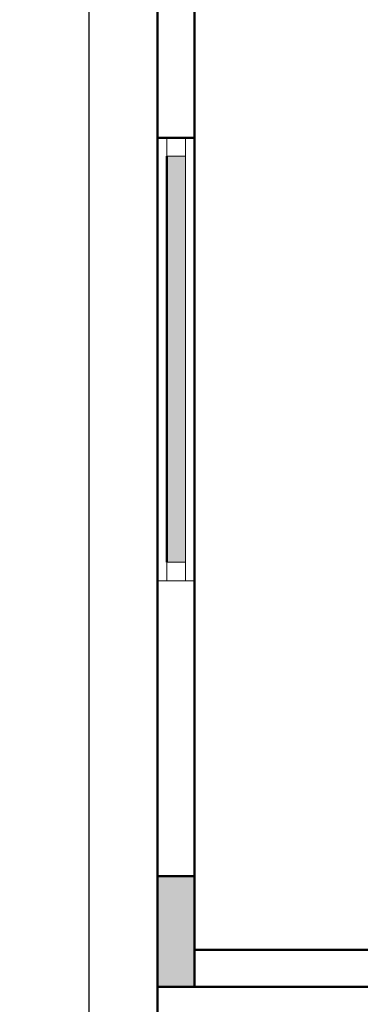
# Model space of a CAD drawing. Units: inches. Extents: x 3064 to 19385, y 846 to 15425.
# Tile 11 of 108: x 3625 to 3680, y 974 to 1134. Entities that reach past the tile are written whole.
import ezdxf

# ---------------------------------------------------------------- set-up
doc = ezdxf.new("R2010")
doc.units = ezdxf.units.IN
for name, color, linetype, lineweight in [('A-ANNO-DIMS', 2, 'Continuous', 18), ('A-COLS', 1, 'Continuous', 35), ('A-GLAZ', 4, 'Continuous', 18), ('A-WALL', 7, 'Continuous', 50)]:
    doc.layers.add(name, color=color, linetype=linetype, lineweight=lineweight)
doc.styles.get("Standard").update_dxf_attribs({"font": 'arial.ttf'})
doc.dimstyles.new('ISO-25', dxfattribs={"dimtxt": 9, "dimasz": 2.5, "dimexe": 1.25, "dimexo": 0.625, "dimtad": 1, "dimdec": 1, "dimlunit": 3, "dimtxsty": 'Standard', "dimcen": 2.5, "dimadec": 0, "dimazin": 0, "dimtfac": 1, "dimtdec": 1, "dimtmove": 0, "dimatfit": 3, "dimfxl": 1, "dimarcsym": 0})

# ---------------------------------------------------------------- blocks, each defined once
blk = doc.blocks.new('*D40')
at = {"layer": 'A-ANNO-DIMS', "color": 0, "lineweight": -2, "transparency": 16777216}
for p, q in [((3646.73, 1396.34), (3634.99, 1396.34)), ((3636.24, 906.84), (3636.24, 1393.84)), ((3646.73, 904.34), (3634.99, 904.34))]:
    blk.add_line(p, q, dxfattribs=at)
at = {"layer": 'A-ANNO-DIMS', "color": 0, "transparency": 16777216}
for points in [[(3635.82, 1393.84), (3636.66, 1393.84), (3636.24, 1396.34)], [(3635.82, 906.84), (3636.66, 906.84), (3636.24, 904.34)]]:
    blk.add_solid(points, dxfattribs=at)
at = {"layer": 'Defpoints', "color": 0, "transparency": 16777216}
for p in [(3636.24, 1396.34), (3647.36, 1396.34), (3647.36, 904.34)]:
    blk.add_point(p, dxfattribs=at)
at = {"layer": 'A-ANNO-DIMS', "color": 0, "transparency": 16777216, "insert": (3631.1, 1150.34), "char_height": 9, "attachment_point": 5, "rotation": 90}
blk.add_mtext("41'", dxfattribs=at)
blk = doc.blocks.new('WIN-1900')
blk.add_line((3, 0), (3, 66))
blk.add_lwpolyline([(3, 66), (0, 66), (0, 69), (3, 69)], close=True)

msp = doc.modelspace()

# ---------------------------------------------------------------- hatches: boundary and pattern name
at = {"layer": 'A-COLS'}
h = msp.add_hatch(color=256, dxfattribs=at)
h.dxf.hatch_style = 1
h.paths.add_polyline_path([(3647.36, 976.34), (3653.36, 976.34), (3653.36, 994.34), (3647.36, 994.34)])
at = {"layer": 'A-GLAZ'}
h = msp.add_hatch(color=256, dxfattribs=at)
h.dxf.hatch_style = 1
h.paths.add_polyline_path([(3648.86, 1045.34), (3651.86, 1045.34), (3651.86, 1111.34), (3648.86, 1111.34)])

# ---------------------------------------------------------------- linework, layer by layer
msp.add_line((3653.36, 1042.34), (3647.36, 1042.34), dxfattribs=at)
msp.add_lwpolyline([(3651.86, 1042.34), (3648.86, 1042.34), (3648.86, 1045.34), (3651.86, 1045.34)], close=True, dxfattribs=at)
at = {"layer": 'A-WALL'}
for p, q in [((3647.36, 1396.34), (3647.36, 976.34)), ((3653.36, 1180.34), (3653.36, 982.34)), ((3653.36, 1114.34), (3647.36, 1114.34)), ((3648.86, 1045.34), (3648.86, 1111.34)), ((3782.36, 982.34), (3653.36, 982.34)), ((3989.36, 976.34), (3647.36, 976.34)), ((3653.36, 976.34), (3647.36, 976.34)), ((3647.36, 976.34), (3647.36, 904.34))]:
    msp.add_line(p, q, dxfattribs=at)
msp.add_lwpolyline([(3653.36, 976.34), (3653.36, 994.34), (3647.36, 994.34), (3647.36, 976.34)], close=True, dxfattribs=at)

# ---------------------------------------------------------------- block references
at = {"layer": 'A-GLAZ'}
msp.add_blockref('WIN-1900', (3648.86, 1045.34), dxfattribs=at)

# ---------------------------------------------------------------- dimensions: what is measured, and where the dimension line sits
at = {"layer": 'A-ANNO-DIMS'}
dim = msp.add_linear_dim(base=(3636.24, 1396.34), p1=(3647.36, 904.34), p2=(3647.36, 1396.34), angle=90, dimstyle='ISO-25', override={"dimclrd": 0, "dimclre": 0, "dimclrt": 0}, dxfattribs=at)
dim.commit()
dim.dimension.update_dxf_attribs({"geometry": '*D40', "text_midpoint": (3631.1, 1150.34)})

doc.saveas('drawing.dxf')
